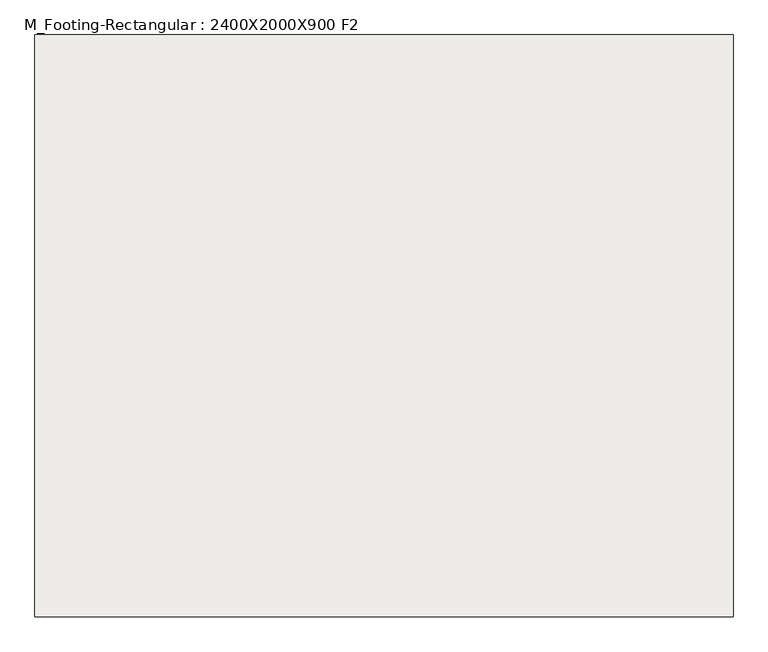
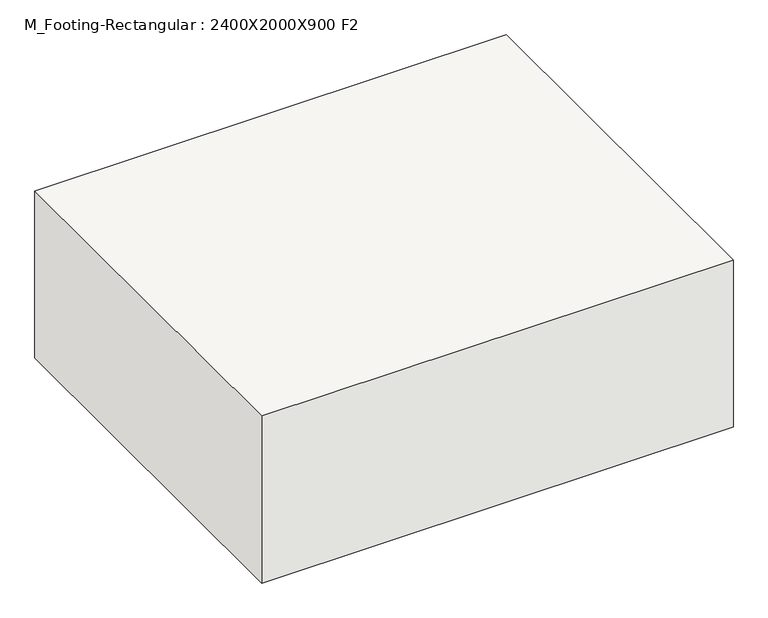
"""IFC4 building model written with IfcOpenShell, lengths in millimetres: slab geometry, M_Footing-Rectangular : 2400X2000X900 F2."""

from ifc_helpers import new_model, si_unit, frame, origin, place, context, project, spatial, polyline, outline, extrude, source, transform, mapped, element, save


def m_footing_rectangular_2400x2000x900_f2_ceb4d106(model_context):
    return source(origin(), model_context, "Body", "SweptSolid", [
        extrude(outline(polyline([(1200.0, 1000.0), (1200.0, -1000.0), (-1200.0, -1000.0), (-1200.0, 1000.0), (1200.0, 1000.0)])), frame((0.0, 0.0, -900.0), z_axis=(0.0, 0.0, 1.0), x_axis=(1.0, 0.0, 0.0)), (0.0, 0.0, 1.0), 900.0),
    ])


if __name__ == "__main__":
    model = new_model("IFC4")
    model_context = context("Model", 3, world=origin())
    ifc_project = project(units=[si_unit("LENGTHUNIT", "METRE", prefix="MILLI")], contexts=[model_context])
    site = spatial("IfcSite", under=ifc_project)
    building = spatial("IfcBuilding", under=site)
    placement = place(None, origin())
    m_footing_rectangular_2400x2000x900_f2_shape = m_footing_rectangular_2400x2000x900_f2_ceb4d106(model_context)
    element("IfcSlab", 1, ObjectType="M_Footing-Rectangular : 2400X2000X900 F2", at=placement, inside=building, context=model_context, shape_type="MappedRepresentation", body=[
        mapped(m_footing_rectangular_2400x2000x900_f2_shape, transform((0.0, 0.0, 0.0), x_axis=(1.0, 0.0, 0.0), y_axis=(0.0, 1.0, 0.0), z_axis=(0.0, 0.0, 1.0))),
    ])
    save(model, "model.ifc")

# Revit data of these elements
# Type "M_Footing-Rectangular : 2400X2000X900 F2"
#   Width = 2400 mm
#   Length = 2000 mm
#   Foundation Thickness = 900 mm
#   Structural Material [instance default] = Concrete, Cast-in-Place gray
#   Assembly Code = ""
# Element 1 (IfcSlab, "M_Footing-Rectangular : 2400X2000X900 F2")
#   Structural Material = Concrete, Cast In Situ
#   Materials on its faces: "Concrete, Cast In Situ"
# Materials
#   "Concrete, Cast-in-Place gray": class "Concrete", colour RGB 192 192 192, transparency 0, Description = "Cast-in-place concrete", Cost = 0
#   "Concrete, Cast In Situ": class "Concrete", colour RGB 192 192 192, transparency 0, Description = "physical material", Cost = 0
